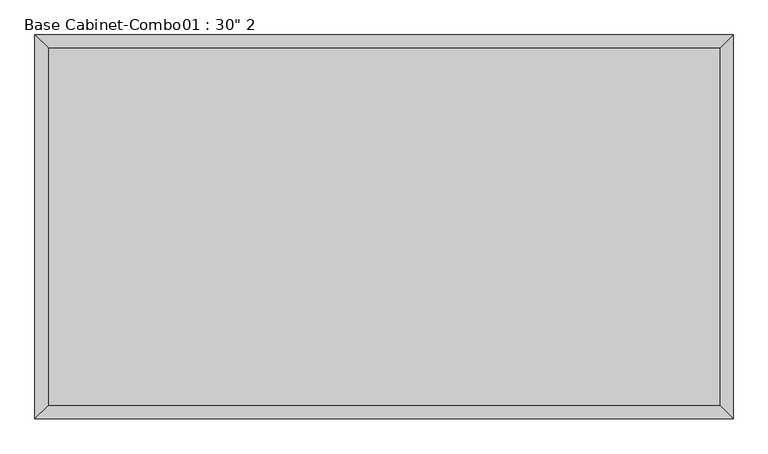
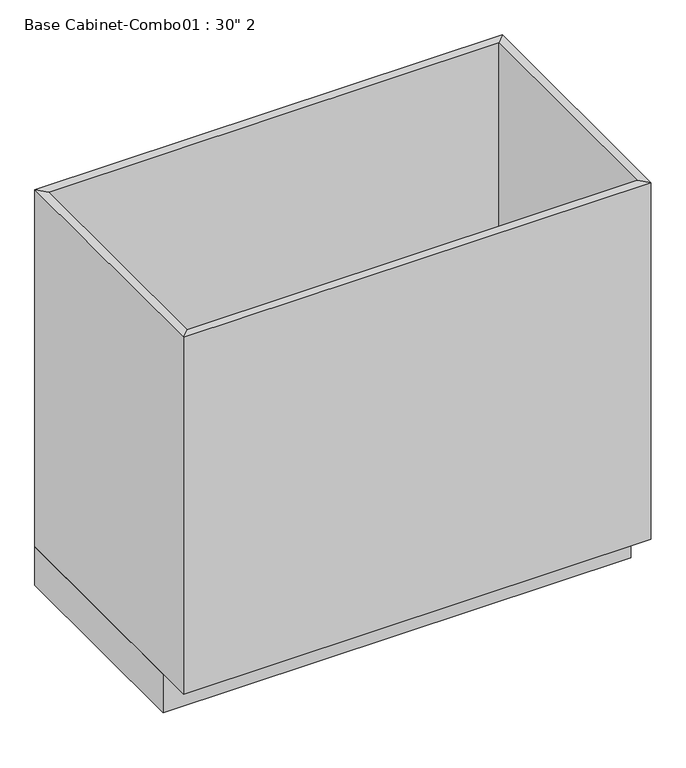
"""IFC4 building model written with IfcOpenShell, lengths in millimetres: furniture geometry."""

from ifc_helpers import new_model, si_unit, frame, origin, origin_with_axes, place, context, project, spatial, polyline, outline, extrude, faceted_brep, source, transform, mapped, element, save


def furniture_5ca60c7f(model_context):
    return source(origin(), model_context, "Body", "SolidModel", [
        extrude(outline(polyline([(526.7377049, 0.0), (526.7377049, -482.6), (-489.2622951, -482.6), (-489.2622951, 0.0), (526.7377049, 0.0)])), origin_with_axes(), (0.0, 0.0, 1.0), 88.9),
        faceted_brep([(507.6877049, -539.75, 908.05), (507.6877049, -539.75, 88.9), (-470.2122951, -539.75, 88.9), (-470.2122951, -539.75, 908.05), (526.7377049, -558.8, 908.05), (-489.2622951, -558.8, 908.05), (526.7377049, -558.8, 88.9), (-489.2622951, -558.8, 88.9), (-470.2122951, -19.05, 88.9), (-470.2122951, -19.05, 908.05), (-489.2622951, 0.0, 908.05), (-489.2622951, 0.0, 88.9), (507.6877049, -19.05, 88.9), (507.6877049, -19.05, 908.05), (526.7377049, 0.0, 908.05), (526.7377049, 0.0, 88.9)], [[[0, 1, 2, 3]], [[4, 0, 3, 5]], [[6, 4, 5, 7]], [[1, 6, 7, 2]], [[3, 2, 8, 9]], [[5, 3, 9, 10]], [[7, 5, 10, 11]], [[2, 7, 11, 8]], [[9, 8, 12, 13]], [[10, 9, 13, 14]], [[11, 10, 14, 15]], [[8, 11, 15, 12]], [[13, 12, 1, 0]], [[14, 13, 0, 4]], [[15, 14, 4, 6]], [[12, 15, 6, 1]]]),
        extrude(outline(polyline([(507.6877049, -19.05), (507.6877049, -539.75), (-470.2122951, -539.75), (-470.2122951, -19.05), (507.6877049, -19.05)])), frame((0.0, 0.0, 88.9), z_axis=(0.0, 0.0, 1.0), x_axis=(1.0, 0.0, 0.0)), (0.0, 0.0, 1.0), 19.05),
    ])


if __name__ == "__main__":
    model = new_model("IFC4")
    model_context = context("Model", 3, world=origin())
    ifc_project = project(units=[si_unit("LENGTHUNIT", "METRE", prefix="MILLI")], contexts=[model_context])
    site = spatial("IfcSite", under=ifc_project)
    building = spatial("IfcBuilding", under=site)
    placement = place(None, origin())
    furniture_shape = furniture_5ca60c7f(model_context)
    element("IfcFurniture", 1, ObjectType="Base Cabinet-Combo01 : 30\" 2", at=placement, inside=building, context=model_context, shape_type="MappedRepresentation", body=[
        mapped(furniture_shape, transform((0.0, 0.0, 0.0), x_axis=(1.0, 0.0, 0.0), y_axis=(0.0, 1.0, 0.0), z_axis=(0.0, 0.0, 1.0))),
    ])
    save(model, "model.ifc")

# Revit data of these elements
# Type "Base Cabinet-Combo01 : 30\" 2"
#   Depth = 1' - 10"
#   Height = 2' - 11 3/4"
#   Toe Depth = 0' - 3"
#   Toe Height = 0' - 3 1/2"
#   Width = 3' - 4"
#   Default Elevation = 0
# Element 1 (IfcFurniture, "Base Cabinet-Combo01 : 30\" 2")
#   Materials on its faces: "Cabinet"
# Materials
#   "Cabinet": colour RGB 204 122 2, transparency 0
